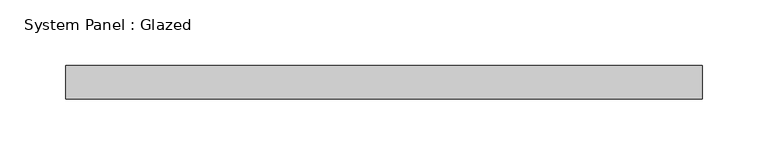
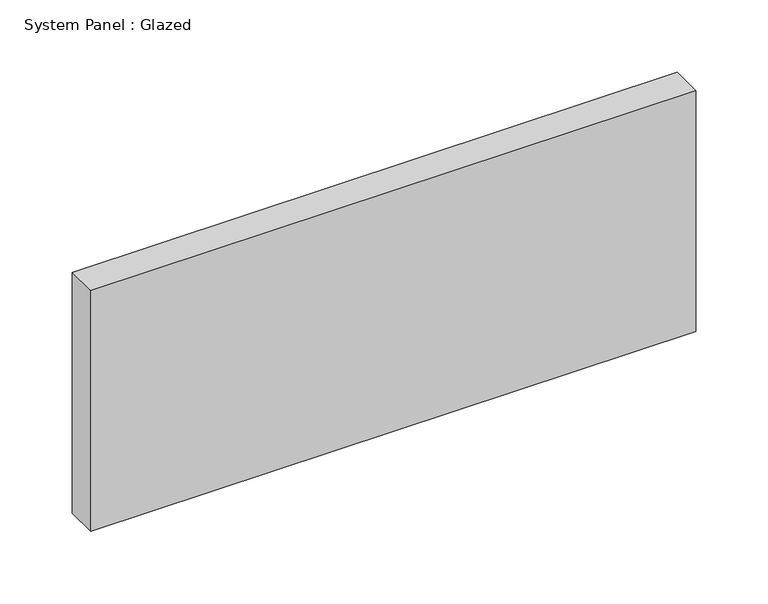
"""IFC4 building model written with IfcOpenShell, lengths in millimetres: plate geometry, System Panel : Glazed."""

from ifc_helpers import new_model, si_unit, origin, origin_with_axes, place, context, project, spatial, polyline, outline, extrude, source, transform, mapped, element, save


def system_panel_glazed_9eb8e914(model_context):
    return source(origin(), model_context, "Body", "SweptSolid", [
        extrude(outline(polyline([(241.3, 19.05), (-241.3, 19.05), (-241.3, 44.45), (241.3, 44.45), (241.3, 19.05)])), origin_with_axes(), (0.0, 0.0, 1.0), 203.2),
    ])


if __name__ == "__main__":
    model = new_model("IFC4")
    model_context = context("Model", 3, world=origin())
    ifc_project = project(units=[si_unit("LENGTHUNIT", "METRE", prefix="MILLI")], contexts=[model_context])
    site = spatial("IfcSite", under=ifc_project)
    building = spatial("IfcBuilding", under=site)
    placement = place(None, origin())
    system_panel_glazed_shape = system_panel_glazed_9eb8e914(model_context)
    element("IfcPlate", 1, ObjectType="System Panel : Glazed", at=placement, inside=building, context=model_context, shape_type="MappedRepresentation", body=[
        mapped(system_panel_glazed_shape, transform((0.0, 0.0, 0.0), x_axis=(1.0, 0.0, 0.0), y_axis=(0.0, 1.0, 0.0), z_axis=(0.0, 0.0, 1.0))),
    ])
    save(model, "model.ifc")

# Revit data of these elements
# Type "System Panel : Glazed"
#   Construction Type Id = "GSP4R"
#   Analytic Construction = "1/8 in Pilkington single glazing"
#   Visual Light Transmittance = 0.9
#   Solar Heat Gain Coefficient = 0.86
#   Heat Transfer Coefficient (U) = 1.18115 BTU/(h·ft²·°F)
#   Define Thermal Properties by = 1
# Element 1 (IfcPlate, "System Panel : Glazed")
#   Materials on its faces: "Glass"
# Materials
#   "Glass": class "Glass", colour RGB 0 128 192, transparency 0.75, Description = "Soda Lime Glass", Cost = 0
